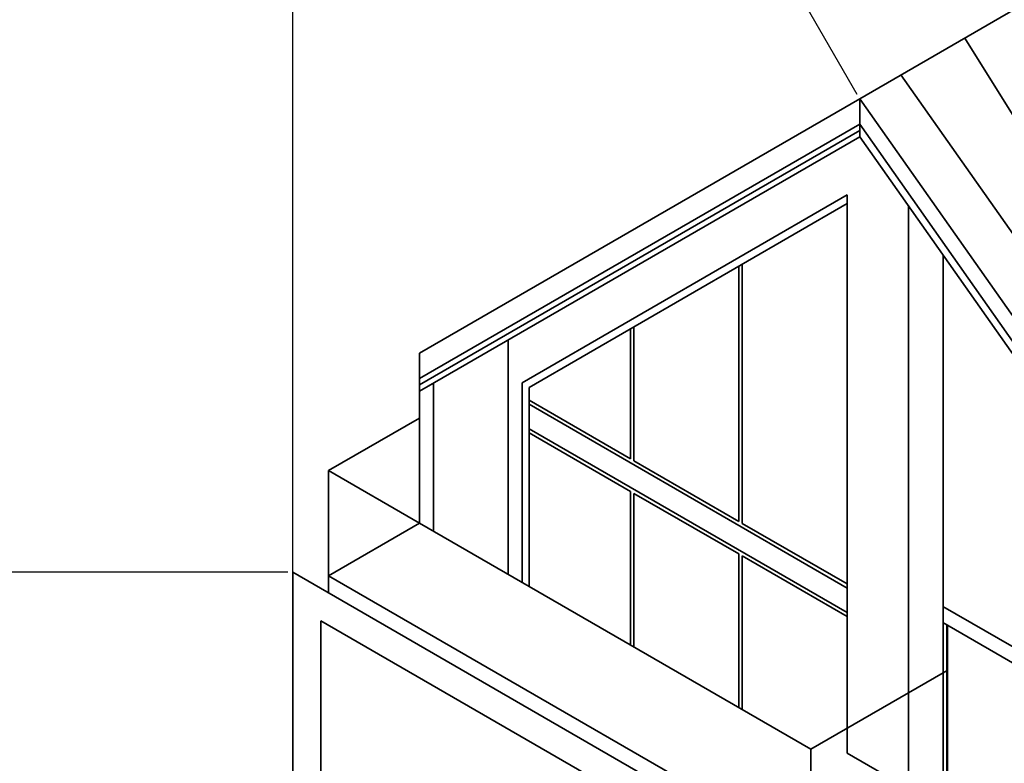
# Model space of a CAD drawing. Units: metres. Extents: x 12735 to 25554, y 20954 to 41989.
# Tile 8 of 15: x 12743.95 to 12756.13, y 20979.54 to 20988.74. Entities that reach past the tile are written whole.
import ezdxf

# ---------------------------------------------------------------- set-up
doc = ezdxf.new("R2010")
doc.units = ezdxf.units.M
doc.layers.get('Defpoints').update_dxf_attribs({"lineweight": 13})
doc.layers.add('A-ANNO-DIMS', color=2, linetype='Continuous', lineweight=18)
doc.layers.add('A-ELEV', color=7, linetype='Continuous', lineweight=35)
doc.styles.get("Standard").update_dxf_attribs({"font": 'arial.ttf'})
doc.dimstyles.get("Standard").update_dxf_attribs({"dimtxt": 0.18, "dimasz": 0.18, "dimexe": 0.18, "dimexo": 0.0625, "dimgap": 0.09, "dimtad": 0, "dimtih": 1, "dimtoh": 1, "dimdec": 4, "dimzin": 0, "dimdsep": 46, "dimtxsty": 'Standard', "dimcen": 0.09, "dimadec": 0, "dimazin": 0, "dimtfac": 1, "dimtdec": 4, "dimtofl": 0, "dimtmove": 0, "dimatfit": 3, "dimfxl": 1, "dimtolj": 1, "dimtzin": 0, "dimarcsym": 0})

# ---------------------------------------------------------------- blocks, each defined once
blk = doc.blocks.new('*D10')
at = {"layer": 'A-ANNO-DIMS', "color": 0, "lineweight": -2, "transparency": 16777216}
for p, q in [((12766.645, 20994.825), (12783.484, 20994.825)), ((12783.304, 20994.645), (12783.304, 20975.781)), ((12783.304, 20956.553), (12783.304, 20975.417)), ((12755.849, 20956.373), (12783.484, 20956.373))]:
    blk.add_line(p, q, dxfattribs=at)
at = {"layer": 'A-ANNO-DIMS', "color": 0, "transparency": 16777216}
for points in [[(12783.274, 20994.645), (12783.334, 20994.645), (12783.304, 20994.825)], [(12783.274, 20956.553), (12783.334, 20956.553), (12783.304, 20956.373)]]:
    blk.add_solid(points, dxfattribs=at)
at = {"layer": 'Defpoints', "color": 0, "transparency": 16777216}
for p in [(12766.582, 20994.825), (12783.304, 20994.825), (12755.787, 20956.373)]:
    blk.add_point(p, dxfattribs=at)
at = {"layer": 'A-ANNO-DIMS', "color": 0, "transparency": 16777216, "insert": (12783.304, 20975.599), "char_height": 0.18, "attachment_point": 5}
blk.add_mtext('\\A1;38.45', dxfattribs=at)
blk = doc.blocks.new('*D17')
at = {"layer": 'A-ANNO-DIMS', "color": 0, "lineweight": -2, "transparency": 16777216}
for p, q in [((12766.606, 20994.911), (12765.397, 20997.004)), ((12765.331, 20996.758), (12759.656, 20993.482)), ((12753.351, 20989.842), (12759.026, 20993.118)), ((12754.314, 20987.814), (12753.105, 20989.908))]:
    blk.add_line(p, q, dxfattribs=at)
at = {"layer": 'A-ANNO-DIMS', "color": 0, "transparency": 16777216}
for points in [[(12765.316, 20996.784), (12765.346, 20996.732), (12765.487, 20996.848)], [(12753.336, 20989.868), (12753.366, 20989.816), (12753.195, 20989.752)]]:
    blk.add_solid(points, dxfattribs=at)
at = {"layer": 'Defpoints', "color": 0, "transparency": 16777216}
for p in [(12765.487, 20996.848), (12766.637, 20994.856), (12754.345, 20987.76)]:
    blk.add_point(p, dxfattribs=at)
at = {"layer": 'A-ANNO-DIMS', "color": 0, "transparency": 16777216, "insert": (12759.341, 20993.3), "char_height": 0.18, "attachment_point": 5}
blk.add_mtext('\\A1;14.193', dxfattribs=at)
blk = doc.blocks.new('*D19')
at = {"layer": 'A-ANNO-DIMS', "color": 0, "lineweight": -2, "transparency": 16777216}
for p, q in [((12747.33, 20976.079), (12747.33, 20997.336)), ((12773.306, 20974.774), (12773.306, 20997.336)), ((12747.51, 20997.156), (12759.853, 20997.156)), ((12773.126, 20997.156), (12760.783, 20997.156))]:
    blk.add_line(p, q, dxfattribs=at)
at = {"layer": 'A-ANNO-DIMS', "color": 0, "transparency": 16777216}
for points in [[(12747.51, 20997.186), (12747.51, 20997.126), (12747.33, 20997.156)], [(12773.126, 20997.186), (12773.126, 20997.126), (12773.306, 20997.156)]]:
    blk.add_solid(points, dxfattribs=at)
at = {"layer": 'Defpoints', "color": 0, "transparency": 16777216}
for p in [(12773.306, 20997.156), (12747.33, 20976.016), (12773.306, 20974.711)]:
    blk.add_point(p, dxfattribs=at)
at = {"layer": 'A-ANNO-DIMS', "color": 0, "transparency": 16777216, "insert": (12760.318, 20997.156), "char_height": 0.18, "attachment_point": 5}
blk.add_mtext('\\A1;25.976', dxfattribs=at)
blk = doc.blocks.new('*D20')
at = {"layer": 'A-ANNO-DIMS', "color": 0, "lineweight": -2, "transparency": 16777216}
for p, q in [((12747.267, 20981.902), (12735.363, 20981.902)), ((12735.543, 20981.722), (12735.543, 20979.141)), ((12735.543, 20976.196), (12735.543, 20978.777)), ((12747.267, 20976.016), (12735.363, 20976.016))]:
    blk.add_line(p, q, dxfattribs=at)
at = {"layer": 'A-ANNO-DIMS', "color": 0, "transparency": 16777216}
for points in [[(12735.513, 20981.722), (12735.573, 20981.722), (12735.543, 20981.902)], [(12735.513, 20976.196), (12735.573, 20976.196), (12735.543, 20976.016)]]:
    blk.add_solid(points, dxfattribs=at)
at = {"layer": 'Defpoints', "color": 0, "transparency": 16777216}
for p in [(12747.33, 20981.902), (12735.543, 20976.016), (12747.33, 20976.016)]:
    blk.add_point(p, dxfattribs=at)
at = {"layer": 'A-ANNO-DIMS', "color": 0, "transparency": 16777216, "insert": (12735.543, 20978.959), "char_height": 0.18, "attachment_point": 5}
blk.add_mtext('\\A1;5.886', dxfattribs=at)

msp = doc.modelspace()

# ---------------------------------------------------------------- linework, layer by layer
at = {"layer": 'A-ELEV'}
for p, q in [((12754.3454, 20987.7599), (12766.637, 20994.8564)), ((12760.6982, 20980.3905), (12755.6472, 20988.5115)), ((12754.8551, 20988.0542), (12760.3792, 20980.2064)), ((12748.8963, 20984.6138), (12754.3454, 20987.7599)), ((12754.3454, 20987.4453), (12754.3454, 20987.7599)), ((12754.3454, 20987.7599), (12759.8695, 20979.9121)), ((12748.8963, 20984.2992), (12754.3454, 20987.4453)), ((12754.3454, 20987.4453), (12754.3454, 20987.3662)), ((12754.3454, 20987.4453), (12754.3454, 20987.2893)), ((12754.3454, 20987.4453), (12759.8725, 20979.5932)), ((12748.8963, 20984.2201), (12754.3454, 20987.3662)), ((12754.3454, 20987.2893), (12748.8963, 20984.1432)), ((12754.3454, 20987.2893), (12759.8695, 20979.4415)), ((12750.1661, 20984.2472), (12754.1896, 20986.5702)), ((12754.1896, 20986.5702), (12754.1896, 20979.6647)), ((12750.2527, 20984.1891), (12754.1896, 20986.4621)), ((12754.951, 20986.429), (12754.951, 20979.2251)), ((12755.379, 20985.821), (12755.379, 20979.4722)), ((12752.8485, 20985.6878), (12752.8485, 20982.5309)), ((12752.8918, 20985.7128), (12752.8918, 20982.5059)), ((12751.5073, 20984.9134), (12751.5073, 20983.3053)), ((12751.5506, 20984.9384), (12751.5506, 20983.2803)), ((12749.9929, 20981.8758), (12749.9929, 20984.7764)), ((12748.8963, 20984.6138), (12748.8963, 20984.1432)), ((12748.8963, 20984.1432), (12749.0695, 20984.2432)), ((12749.0695, 20982.409), (12749.0695, 20984.2432)), ((12750.1661, 20981.7758), (12750.1661, 20984.2472)), ((12750.2527, 20981.7258), (12750.2527, 20984.1891)), ((12748.8963, 20982.509), (12748.8963, 20984.1432)), ((12750.2527, 20984.0296), (12751.5073, 20983.3053)), ((12750.2527, 20983.9796), (12754.1896, 20981.7066)), ((12747.7704, 20983.159), (12748.8963, 20983.809)), ((12750.2527, 20983.6769), (12754.1896, 20981.4039)), ((12750.2527, 20983.6269), (12751.5073, 20982.9025)), ((12751.5506, 20983.2803), (12752.8485, 20982.5309)), ((12755.379, 20980.6585), (12755.379, 20983.1904)), ((12747.7704, 20981.859), (12747.7704, 20983.159)), ((12747.7704, 20983.159), (12748.8963, 20982.509)), ((12751.5073, 20982.9025), (12751.5073, 20981.0015)), ((12751.5506, 20982.8775), (12751.5506, 20980.9765)), ((12751.5506, 20982.8775), (12752.8485, 20982.1282)), ((12747.7704, 20981.859), (12748.8963, 20982.509)), ((12748.8963, 20982.509), (12753.7402, 20979.7124)), ((12752.8918, 20982.5059), (12754.1896, 20981.7566)), ((12752.8485, 20982.1282), (12752.8485, 20980.2272)), ((12752.8918, 20982.1032), (12752.8918, 20980.2022)), ((12752.8918, 20982.1032), (12754.1896, 20981.3539)), ((12753.7402, 20978.2012), (12747.3297, 20981.9023)), ((12747.3297, 20981.9023), (12747.3297, 20976.0163)), ((12747.7704, 20981.6478), (12747.7704, 20981.859)), ((12747.7704, 20981.859), (12753.7402, 20978.4124)), ((12755.3743, 20981.4792), (12759.8671, 20978.8853)), ((12753.7402, 20977.8012), (12747.6761, 20981.3023)), ((12747.6761, 20981.3023), (12747.6761, 20976.2163)), ((12755.3743, 20981.2792), (12759.8671, 20978.6853)), ((12755.4237, 20979.1215), (12755.4237, 20981.2507)), ((12755.4323, 20979.1165), (12755.4323, 20981.2457)), ((12753.7402, 20979.7124), (12755.379, 20980.6585)), ((12755.379, 20980.6585), (12755.4284, 20980.687)), ((12755.379, 20979.1473), (12755.379, 20980.6585)), ((12753.7402, 20978.2012), (12753.7402, 20979.7124)), ((12754.951, 20979.2251), (12754.1896, 20979.6647))]:
    msp.add_line(p, q, dxfattribs=at)
at = {"layer": 'Defpoints'}
for p in [(12752.8485, 20985.7959), (12751.5073, 20985.0216)]:
    msp.add_point(p, dxfattribs=at)

# ---------------------------------------------------------------- dimensions: what is measured, and where the dimension line sits
at = {"layer": 'A-ANNO-DIMS'}
dim = msp.add_linear_dim(base=(12773.3057, 20997.1564), p1=(12747.3297, 20976.0163), p2=(12773.3057, 20974.7113), dimstyle='Standard', override={"dimdec": 3, "dimlfac": 1, "dimrnd": 0, "dimzin": 0, "dimdsep": 46, "dimlunit": 2}, dxfattribs=at)
dim.commit()
dim.dimension.update_dxf_attribs({"geometry": '*D19', "text_midpoint": (12760.3177, 20997.1564)})
for base, p1, p2, angle, override, picture, middle in [((12765.487, 20996.8483), (12754.3454, 20987.7599), (12766.637, 20994.8564), 30, {"dimdec": 3, "dimlfac": 1, "dimrnd": 0, "dimzin": 0, "dimdsep": 46, "dimlunit": 2}, '*D17', (12759.3412, 20993.3)), ((12783.3041, 20994.8247), (12755.7869, 20956.3734), (12766.582, 20994.8247), 90, {"dimdec": 2, "dimlfac": 1, "dimrnd": 0, "dimzin": 0, "dimdsep": 46, "dimlunit": 2}, '*D10', (12783.3041, 20975.599)), ((12735.5426, 20976.0163), (12747.3297, 20981.9023), (12747.3297, 20976.0163), 90, {"dimdec": 3, "dimlfac": 1, "dimrnd": 0, "dimzin": 0, "dimdsep": 46, "dimlunit": 2}, '*D20', (12735.5426, 20978.9593))]:
    dim = msp.add_linear_dim(base=base, p1=p1, p2=p2, angle=angle, dimstyle='Standard', override=override, dxfattribs=at)
    dim.commit()
    dim.dimension.update_dxf_attribs({"geometry": picture, "text_midpoint": middle})

doc.saveas('drawing.dxf')
